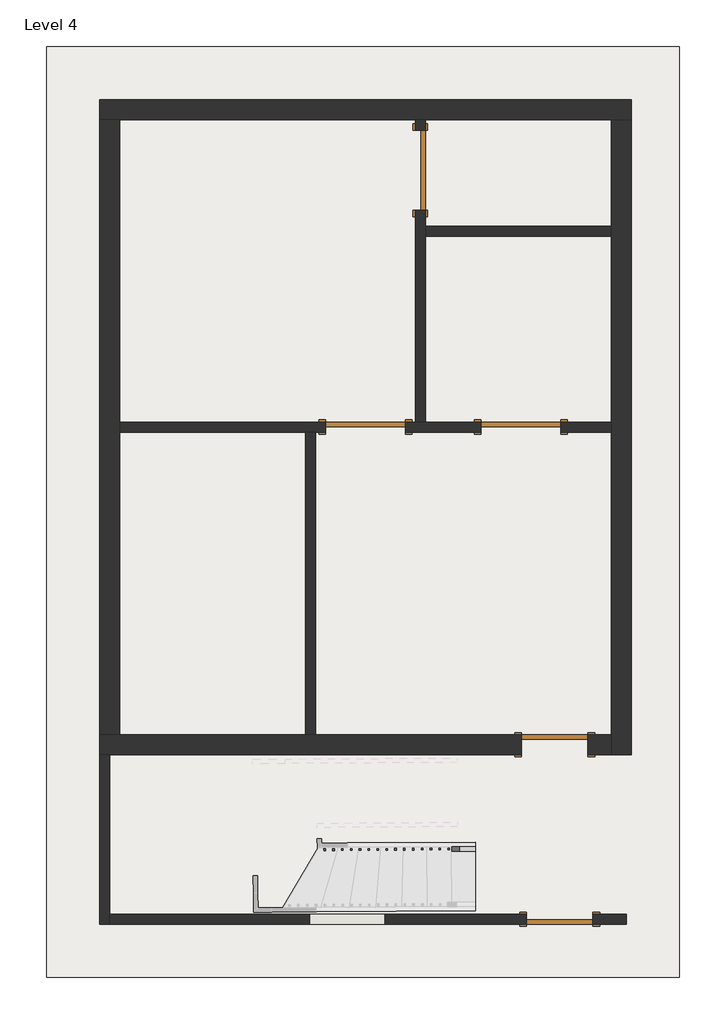
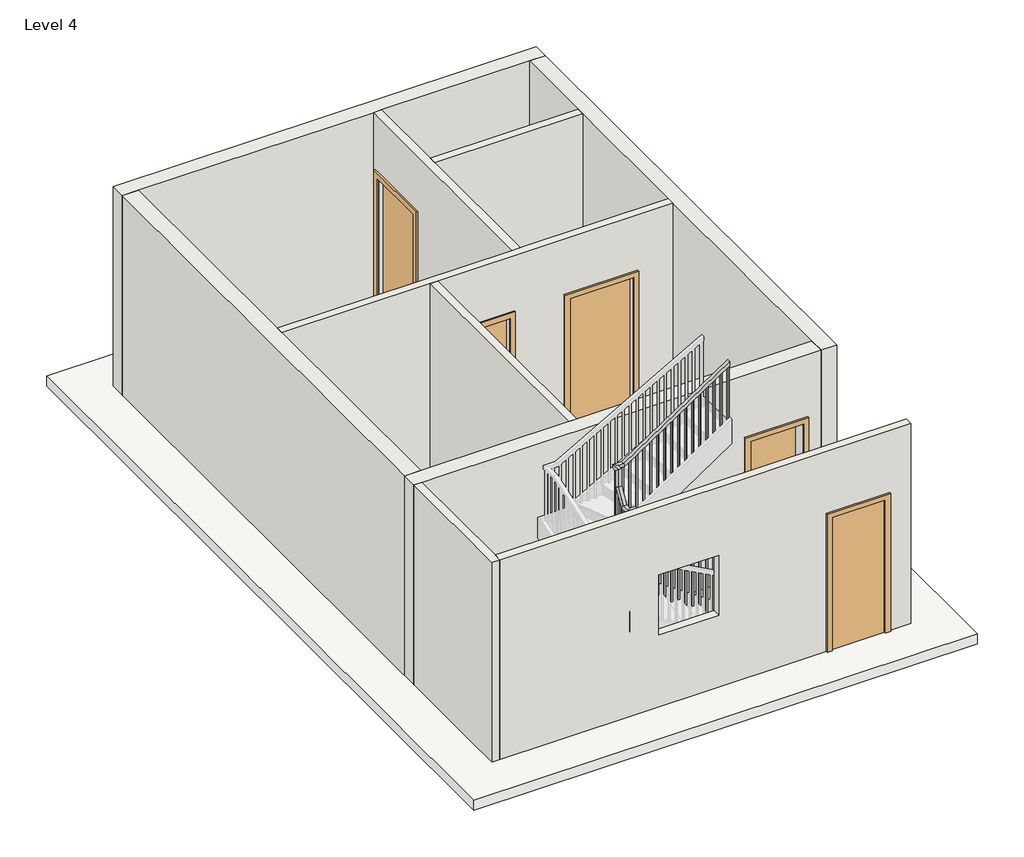
# One storey, part 1 of 2: 10 walls, 5 doors, 1 railing, 1 roof.
"""IFC4 building model written with IfcOpenShell, lengths in millimetres."""

from ifc_helpers import new_model, si_unit, frame, origin, place, context, project, spatial, polyline, outline, extrude, faceted_brep, transform, mapped, element, save
from components import door_a1484949, door_d8f5dbb5, door_e5f9f3c4, door_305aa2a5

model = new_model("IFC4")

# Units and contexts
model_context = context("Model", 3, world=origin())
ifc_project = project(units=[si_unit("LENGTHUNIT", "METRE", prefix="MILLI")], contexts=[model_context])

# Site, building, storey
site = spatial("IfcSite", under=ifc_project)
building = spatial("IfcBuilding", under=site)
storey = spatial("IfcBuildingStorey", under=building, Name="Level 4", Elevation=6400.8)

# Doors
placement = place(None, origin())
door_shape = door_a1484949(model_context)
element("IfcDoor", 1, ObjectType="Single-Flush : 30\" x 80\"", at=placement, inside=storey, context=model_context, shape_type="MappedRepresentation", body=[
    mapped(door_shape, transform((792.5410386, -2372.0109248, 6400.8), x_axis=(1.0, 0.0, 0.0), y_axis=(0.0, 1.0, 0.0), z_axis=(0.0, 0.0, 1.0))),
])
door_2_shape = door_d8f5dbb5(model_context)
element("IfcDoor", 2, ObjectType="Single-Flush : 30\" x 80\"", at=placement, inside=storey, context=model_context, shape_type="MappedRepresentation", body=[
    mapped(door_2_shape, transform((849.6910386, -4372.2609248, 6400.8), x_axis=(-1.0, 0.0, 0.0), y_axis=(0.0, -1.0, 0.0), z_axis=(0.0, 0.0, 1.0))),
])
door_3_shape = door_e5f9f3c4(model_context)
element("IfcDoor", 3, ObjectType="Single-Flush : 36\" x 84\"", at=placement, inside=storey, context=model_context, shape_type="MappedRepresentation", body=[
    mapped(door_3_shape, transform((-750.5089614, 4209.7640752, 6400.8), x_axis=(0.0, -1.0, 0.0), y_axis=(1.0, 0.0, 0.0), z_axis=(0.0, 0.0, 1.0))),
])
door_4_shape = door_305aa2a5(model_context)
element("IfcDoor", 4, ObjectType="Single-Flush : 36\" x 84\"", at=placement, inside=storey, context=model_context, shape_type="MappedRepresentation", body=[
    mapped(door_4_shape, transform((402.0160386, 1266.5390752, 6400.8), x_axis=(-1.0, 0.0, 0.0), y_axis=(0.0, -1.0, 0.0), z_axis=(0.0, 0.0, 1.0))),
])
element("IfcDoor", 5, ObjectType="Single-Flush : 36\" x 84\"", at=placement, inside=storey, context=model_context, shape_type="MappedRepresentation", body=[
    mapped(door_4_shape, transform((-1379.1589614, 1266.5390752, 6400.8), x_axis=(-1.0, 0.0, 0.0), y_axis=(0.0, -1.0, 0.0), z_axis=(0.0, 0.0, 1.0))),
])

# Railing
element("IfcRailing", 6, ObjectType="Handrail - Rectangular", at=placement, inside=storey, context=model_context, shape_type="SolidModel", body=[
    faceted_brep([(-120.3816305, -3590.4209536, 7484.5333333), (-120.3816305, -3590.4209536, 7423.3630107), (-120.6930289, -3539.621908, 7423.3630107), (-120.6930289, -3539.621908, 7484.5333333), (-1854.5612186, -3601.0514854, 8647.8182998), (-1905.3602642, -3601.3628839, 8620.7238978), (-1905.6716627, -3550.5638383, 8620.7238978), (-1854.8726171, -3550.2524399, 8647.8182998), (-1854.5612186, -3601.0514854, 8870.0829276), (-1905.3602642, -3601.3628839, 8819.2829276), (-1905.6716627, -3550.5638383, 8819.2829276), (-1854.8726171, -3550.2524399, 8870.0829276), (-1981.5588325, -3601.8299816, 8870.0829276), (-1981.5588325, -3601.8299816, 8819.2829276), (-1931.0711854, -3550.7195376, 8819.2829276), (-1931.0711854, -3550.7195376, 8870.0829276), (-1982.3373287, -3474.8323677, 8870.0829276), (-1982.5128182, -3446.2044317, 8819.2829276), (-1931.7137726, -3445.8930332, 8819.2829276), (-1931.5382832, -3474.5209692, 8870.0829276), (-1983.1158249, -3347.8347538, 9079.8434812), (-1983.4272234, -3297.0357082, 9065.6632575), (-1932.6281778, -3296.7243097, 9065.6632575), (-1932.3167793, -3347.5233553, 9079.8434812), (-1983.1158249, -3347.8347538, 9351.2951436), (-1983.4272234, -3297.0357082, 9300.4951436), (-1932.6281778, -3296.7243097, 9300.4951436), (-1932.3167793, -3347.5233553, 9351.2951436), (-1983.8943211, -3220.8371398, 9351.2951436), (-1983.8943211, -3220.8371398, 9300.4951436), (-1932.783877, -3271.3247869, 9300.4951436), (-1932.783877, -3271.3247869, 9351.2951436), (-1856.8967072, -3220.0586437, 9351.2951436), (-1841.6341703, -3219.9650842, 9300.4951436), (-1841.3227719, -3270.7641298, 9300.4951436), (-1856.5853087, -3270.8576892, 9351.2951436), (-324.9523945, -3210.6678153, 10363.2), (-324.6409961, -3261.4668609, 10363.2), (-324.6409961, -3261.4668609, 10302.3185401), (-324.9523945, -3210.6678153, 10302.3185401)], [[[0, 1, 2, 3]], [[1, 0, 4, 5]], [[2, 1, 5, 6]], [[3, 2, 6, 7]], [[0, 3, 7, 4]], [[5, 4, 8, 9]], [[6, 5, 9, 10]], [[7, 6, 10, 11]], [[4, 7, 11, 8]], [[9, 8, 12, 13]], [[10, 9, 13, 14]], [[11, 10, 14, 15]], [[8, 11, 15, 12]], [[13, 12, 16, 17]], [[14, 13, 17, 18]], [[15, 14, 18, 19]], [[12, 15, 19, 16]], [[17, 16, 20, 21]], [[18, 17, 21, 22]], [[19, 18, 22, 23]], [[16, 19, 23, 20]], [[21, 20, 24, 25]], [[22, 21, 25, 26]], [[23, 22, 26, 27]], [[20, 23, 27, 24]], [[25, 24, 28, 29]], [[26, 25, 29, 30]], [[27, 26, 30, 31]], [[24, 27, 31, 28]], [[29, 28, 32, 33]], [[30, 29, 33, 34]], [[31, 30, 34, 35]], [[28, 31, 35, 32]], [[36, 37, 38, 39]], [[33, 32, 36, 39]], [[34, 33, 39, 38]], [[35, 34, 38, 37]], [[32, 35, 37, 36]]]),
    extrude(outline(polyline([(222.3085098, -19.05), (234.8914903, 0.0), (1246.1854534, 0.0), (1246.1854534, -19.05), (222.3085098, -19.05)])), frame((-342.2360746, -3245.6994205, 10525.6521201), z_axis=(-0.00612989118043648, 0.9999812120405643, 0.0), x_axis=(0.0, 0.0, -1.0)), (0.0, 0.0, 1.0), 19.05),
    extrude(outline(polyline([(222.3085098, -19.0499999), (234.8914902, 0.0), (1179.0762243, 0.0), (1179.0762243, -19.0499999), (222.3085098, -19.0499999)])), frame((-443.8341657, -3246.3222175, 10458.542891), z_axis=(-0.00612989118043648, 0.9999812120405643, 0.0), x_axis=(0.0, 0.0, -1.0)), (0.0, 0.0, 1.0), 19.05),
    extrude(outline(polyline([(222.3085098, -19.05), (234.8914902, 0.0), (1111.9669952, 0.0), (1111.9669952, -19.05), (222.3085098, -19.05)])), frame((-545.4322569, -3246.9450144, 10391.4336619), z_axis=(-0.00612989118043648, 0.9999812120405643, 0.0), x_axis=(0.0, 0.0, -1.0)), (0.0, 0.0, 1.0), 19.05),
    extrude(outline(polyline([(222.3085098, -19.05), (234.8914902, 0.0), (1214.1910995, 0.0), (1214.1910995, -19.05), (222.3085098, -19.05)])), frame((-647.030348, -3247.5678114, 10324.3244328), z_axis=(-0.00612989118043648, 0.9999812120405643, 0.0), x_axis=(0.0, 0.0, -1.0)), (0.0, 0.0, 1.0), 19.05),
    extrude(outline(polyline([(222.3085098, -19.05), (234.8914902, 0.0), (1147.0818704, 0.0), (1147.0818704, -19.05), (222.3085098, -19.05)])), frame((-748.6284392, -3248.1906083, 10257.2152037), z_axis=(-0.00612989118043648, 0.9999812120405643, 0.0), x_axis=(0.0, 0.0, -1.0)), (0.0, 0.0, 1.0), 19.05),
    extrude(outline(polyline([(222.3085098, -19.05), (234.8914902, 0.0), (1079.9726413, 0.0), (1079.9726413, -19.05), (222.3085098, -19.05)])), frame((-850.2265303, -3248.8134053, 10190.1059746), z_axis=(-0.00612989118043648, 0.9999812120405643, 0.0), x_axis=(0.0, 0.0, -1.0)), (0.0, 0.0, 1.0), 19.05),
    extrude(outline(polyline([(222.3085098, -19.05), (234.8914902, 0.0), (1182.1967455, 0.0), (1182.1967455, -19.05), (222.3085098, -19.05)])), frame((-951.8246215, -3249.4362022, 10122.9967455), z_axis=(-0.00612989118043648, 0.9999812120405643, 0.0), x_axis=(0.0, 0.0, -1.0)), (0.0, 0.0, 1.0), 19.05),
    extrude(outline(polyline([(222.3085097, -19.05), (234.8914902, 0.0), (1115.0875164, 0.0), (1115.0875164, -19.05), (222.3085097, -19.05)])), frame((-1053.4227126, -3250.0589992, 10055.8875164), z_axis=(-0.00612989118043648, 0.9999812120405643, 0.0), x_axis=(0.0, 0.0, -1.0)), (0.0, 0.0, 1.0), 19.05),
    extrude(outline(polyline([(222.3085097, -19.0499999), (234.8914902, 0.0), (1047.9782873, 0.0), (1047.9782873, -19.0499999), (222.3085097, -19.0499999)])), frame((-1155.0208037, -3250.6817961, 9988.7782873), z_axis=(-0.00612989118043648, 0.9999812120405643, 0.0), x_axis=(0.0, 0.0, -1.0)), (0.0, 0.0, 1.0), 19.05),
    extrude(outline(polyline([(222.3085097, -19.05), (234.8914902, 0.0), (1150.2023915, 0.0), (1150.2023915, -19.05), (222.3085097, -19.05)])), frame((-1256.6188949, -3251.304593, 9921.6690582), z_axis=(-0.00612989118043648, 0.9999812120405643, 0.0), x_axis=(0.0, 0.0, -1.0)), (0.0, 0.0, 1.0), 19.05),
    extrude(outline(polyline([(222.3085098, -19.05), (234.8914903, 0.0), (1083.0931625, 0.0), (1083.0931625, -19.05), (222.3085098, -19.05)])), frame((-1358.216986, -3251.92739, 9854.5598292), z_axis=(-0.00612989118043648, 0.9999812120405643, 0.0), x_axis=(0.0, 0.0, -1.0)), (0.0, 0.0, 1.0), 19.05),
    extrude(outline(polyline([(222.3085098, -19.05), (234.8914903, 0.0), (1185.3172668, 0.0), (1185.3172668, -19.05), (222.3085098, -19.05)])), frame((-1459.8150772, -3252.5501869, 9787.4506001), z_axis=(-0.00612989118043648, 0.9999812120405643, 0.0), x_axis=(0.0, 0.0, -1.0)), (0.0, 0.0, 1.0), 19.05),
    extrude(outline(polyline([(222.3085098, -19.05), (234.8914903, 0.0), (1118.2080377, 0.0), (1118.2080377, -19.05), (222.3085098, -19.05)])), frame((-1561.4131683, -3253.1729839, 9720.341371), z_axis=(-0.00612989118043648, 0.9999812120405643, 0.0), x_axis=(0.0, 0.0, -1.0)), (0.0, 0.0, 1.0), 19.05),
    extrude(outline(polyline([(222.3085098, -19.05), (234.8914902, 0.0), (1051.0988086, 0.0), (1051.0988086, -19.05), (222.3085098, -19.05)])), frame((-1663.0112595, -3253.7957808, 9653.2321419), z_axis=(-0.00612989118043648, 0.9999812120405643, 0.0), x_axis=(0.0, 0.0, -1.0)), (0.0, 0.0, 1.0), 19.05),
    extrude(outline(polyline([(222.3085098, -19.05), (234.8914902, 0.0), (1153.3229128, 0.0), (1153.3229128, -19.05), (222.3085098, -19.05)])), frame((-1764.6093506, -3254.4185778, 9586.1229128), z_axis=(-0.00612989118043648, 0.9999812120405643, 0.0), x_axis=(0.0, 0.0, -1.0)), (0.0, 0.0, 1.0), 19.05),
    extrude(outline(polyline([(222.3085098, -19.05), (234.8914902, 0.0), (1086.2136837, 0.0), (1086.2136837, -19.05), (222.3085098, -19.05)])), frame((-1866.2074418, -3255.0413747, 9519.0136837), z_axis=(-0.00612989118043648, 0.9999812120405643, 0.0), x_axis=(0.0, 0.0, -1.0)), (0.0, 0.0, 1.0), 19.05),
    extrude(outline(polyline([(-1948.6001916, -3280.94692), (-1967.6498337, -3281.0636944), (-1967.7666081, -3262.0140523), (-1948.716966, -3261.8972779), (-1948.6001916, -3280.94692)])), frame((0.0, 0.0, 8263.4666667), z_axis=(0.0, 0.0, 1.0), x_axis=(1.0, 0.0, 0.0)), (0.0, 0.0, 1.0), 1037.0284769),
    extrude(outline(polyline([(244.3320415, -19.05), (212.8679585, 0.0), (1074.2735921, 0.0), (1074.2735921, -19.05), (244.3320415, -19.05)])), frame((-1967.1438111, -3363.6121435, 9168.4069254), z_axis=(0.9999812120405644, 0.006129891180436036, 0.0), x_axis=(0.0, 0.0, -1.0)), (0.0, 0.0, 1.0), 19.05),
    extrude(outline(polyline([(244.3320415, -19.05), (212.8679585, 0.0), (1075.7984825, 0.0), (1075.7984825, -19.05), (244.3320415, -19.05)])), frame((-1966.5210142, -3465.2102346, 9000.5984825), z_axis=(0.9999812120405644, 0.006129891180436036, 0.0), x_axis=(0.0, 0.0, -1.0)), (0.0, 0.0, 1.0), 19.05),
    extrude(outline(polyline([(-1939.8365364, -3566.6485675), (-1939.719762, -3585.6982096), (-1958.7694041, -3585.814984), (-1958.8861785, -3566.7653419), (-1939.8365364, -3566.6485675)])), frame((0.0, 0.0, 7755.4666667), z_axis=(0.0, 0.0, 1.0), x_axis=(1.0, 0.0, 0.0)), (0.0, 0.0, 1.0), 1063.816261),
    extrude(outline(polyline([(234.9892351, -19.05), (222.2107648, 0.0), (1224.4109792, 0.0), (1224.4109792, -19.05), (234.9892351, -19.05)])), frame((-1857.171313, -3585.1921871, 8810.5443125), z_axis=(-0.006129891180436334, 0.9999812120405643, 0.0), x_axis=(0.0, 0.0, -1.0)), (0.0, 0.0, 1.0), 19.05),
    extrude(outline(polyline([(234.9892352, -19.05), (222.2107649, 0.0), (1156.259138, 0.0), (1156.259138, -19.05), (234.9892352, -19.05)])), frame((-1755.5732218, -3584.5693901, 8742.3924713), z_axis=(-0.006129891180436334, 0.9999812120405643, 0.0), x_axis=(0.0, 0.0, -1.0)), (0.0, 0.0, 1.0), 19.05),
    extrude(outline(polyline([(234.9892351, -19.05), (222.2107649, 0.0), (1257.44063, 0.0), (1257.44063, -19.05), (234.9892351, -19.05)])), frame((-1653.9751307, -3583.9465932, 8674.24063), z_axis=(-0.006129891180436334, 0.9999812120405643, 0.0), x_axis=(0.0, 0.0, -1.0)), (0.0, 0.0, 1.0), 19.05),
    extrude(outline(polyline([(234.9892351, -19.05), (222.2107649, 0.0), (1189.2887887, 0.0), (1189.2887887, -19.05), (234.9892351, -19.05)])), frame((-1552.3770395, -3583.3237962, 8606.0887887), z_axis=(-0.006129891180436334, 0.9999812120405643, 0.0), x_axis=(0.0, 0.0, -1.0)), (0.0, 0.0, 1.0), 19.05),
    extrude(outline(polyline([(234.9892351, -19.05), (222.2107649, 0.0), (1290.4702807, 0.0), (1290.4702807, -19.05), (234.9892351, -19.05)])), frame((-1450.7789484, -3582.7009993, 8537.9369474), z_axis=(-0.006129891180436334, 0.9999812120405643, 0.0), x_axis=(0.0, 0.0, -1.0)), (0.0, 0.0, 1.0), 19.05),
    extrude(outline(polyline([(234.9892351, -19.0499999), (222.2107649, 0.0), (1222.3184394, 0.0), (1222.3184394, -19.0499999), (234.9892351, -19.0499999)])), frame((-1349.1808572, -3582.0782024, 8469.7851061), z_axis=(-0.006129891180436334, 0.9999812120405643, 0.0), x_axis=(0.0, 0.0, -1.0)), (0.0, 0.0, 1.0), 19.05),
    extrude(outline(polyline([(234.9892351, -19.05), (222.2107648, 0.0), (1154.1665981, 0.0), (1154.1665981, -19.05), (234.9892351, -19.05)])), frame((-1247.5827661, -3581.4554054, 8401.6332648), z_axis=(-0.006129891180436334, 0.9999812120405643, 0.0), x_axis=(0.0, 0.0, -1.0)), (0.0, 0.0, 1.0), 19.05),
    extrude(outline(polyline([(234.9892352, -19.05), (222.2107649, 0.0), (1255.3480903, 0.0), (1255.3480903, -19.05), (234.9892352, -19.05)])), frame((-1145.984675, -3580.8326085, 8333.4814236), z_axis=(-0.006129891180436334, 0.9999812120405643, 0.0), x_axis=(0.0, 0.0, -1.0)), (0.0, 0.0, 1.0), 19.05),
    extrude(outline(polyline([(234.9892351, -19.05), (222.2107649, 0.0), (1187.196249, 0.0), (1187.196249, -19.05), (234.9892351, -19.05)])), frame((-1044.3865838, -3580.2098115, 8265.3295823), z_axis=(-0.006129891180436334, 0.9999812120405643, 0.0), x_axis=(0.0, 0.0, -1.0)), (0.0, 0.0, 1.0), 19.05),
    extrude(outline(polyline([(234.9892351, -19.05), (222.2107649, 0.0), (1288.377741, 0.0), (1288.377741, -19.05), (234.9892351, -19.05)])), frame((-942.7884927, -3579.5870146, 8197.177741), z_axis=(-0.006129891180436334, 0.9999812120405643, 0.0), x_axis=(0.0, 0.0, -1.0)), (0.0, 0.0, 1.0), 19.05),
    extrude(outline(polyline([(234.9892351, -19.05), (222.2107649, 0.0), (1220.2258997, 0.0), (1220.2258997, -19.05), (234.9892351, -19.05)])), frame((-841.1904015, -3578.9642176, 8129.0258997), z_axis=(-0.006129891180436334, 0.9999812120405643, 0.0), x_axis=(0.0, 0.0, -1.0)), (0.0, 0.0, 1.0), 19.05),
    extrude(outline(polyline([(234.9892351, -19.05), (222.2107649, 0.0), (1152.0740584, 0.0), (1152.0740584, -19.05), (234.9892351, -19.05)])), frame((-739.5923104, -3578.3414207, 8060.8740584), z_axis=(-0.006129891180436334, 0.9999812120405643, 0.0), x_axis=(0.0, 0.0, -1.0)), (0.0, 0.0, 1.0), 19.05),
    extrude(outline(polyline([(234.9892351, -19.0499999), (222.2107648, 0.0), (1253.2555504, 0.0), (1253.2555504, -19.0499999), (234.9892351, -19.0499999)])), frame((-637.9942192, -3577.7186237, 7992.7222171), z_axis=(-0.006129891180436334, 0.9999812120405643, 0.0), x_axis=(0.0, 0.0, -1.0)), (0.0, 0.0, 1.0), 19.05),
    extrude(outline(polyline([(234.9892352, -19.05), (222.2107649, 0.0), (1185.1037092, 0.0), (1185.1037092, -19.05), (234.9892352, -19.05)])), frame((-536.3961281, -3577.0958268, 7924.5703759), z_axis=(-0.006129891180436334, 0.9999812120405643, 0.0), x_axis=(0.0, 0.0, -1.0)), (0.0, 0.0, 1.0), 19.05),
    extrude(outline(polyline([(234.9892351, -19.05), (222.2107649, 0.0), (1116.9518679, 0.0), (1116.9518679, -19.05), (234.9892351, -19.05)])), frame((-434.798037, -3576.4730299, 7856.4185346), z_axis=(-0.006129891180436334, 0.9999812120405643, 0.0), x_axis=(0.0, 0.0, -1.0)), (0.0, 0.0, 1.0), 19.05),
    extrude(outline(polyline([(234.9892351, -19.05), (222.2107649, 0.0), (1218.13336, 0.0), (1218.13336, -19.05), (234.9892351, -19.05)])), frame((-333.1999458, -3575.8502329, 7788.2666933), z_axis=(-0.006129891180436334, 0.9999812120405643, 0.0), x_axis=(0.0, 0.0, -1.0)), (0.0, 0.0, 1.0), 19.05),
    extrude(outline(polyline([(234.9892351, -19.05), (222.2107649, 0.0), (1149.9815187, 0.0), (1149.9815187, -19.05), (234.9892351, -19.05)])), frame((-231.6018547, -3575.227436, 7720.114852), z_axis=(-0.006129891180436334, 0.9999812120405643, 0.0), x_axis=(0.0, 0.0, -1.0)), (0.0, 0.0, 1.0), 19.05),
    extrude(outline(polyline([(-1948.7558908, -3255.5473972), (-1967.8055329, -3255.6641716), (-1967.9223073, -3236.6145296), (-1948.8726652, -3236.4977551), (-1948.7558908, -3255.5473972)])), frame((0.0, 0.0, 8263.4666667), z_axis=(0.0, 0.0, 1.0), x_axis=(1.0, 0.0, 0.0)), (0.0, 0.0, 1.0), 1037.0284769),
    extrude(outline(polyline([(-1946.8485752, -3566.6915513), (-1946.7318007, -3585.7411934), (-1965.7814428, -3585.8579679), (-1965.8982173, -3566.8083258), (-1946.8485752, -3566.6915513)])), frame((0.0, 0.0, 7755.4666667), z_axis=(0.0, 0.0, 1.0), x_axis=(1.0, 0.0, 0.0)), (0.0, 0.0, 1.0), 1063.816261),
    extrude(outline(polyline([(222.3085098, -19.05), (234.8914902, 0.0), (1245.1603832, 0.0), (1245.1603832, -19.05), (222.3085098, -19.05)])), frame((-343.7879502, -3245.7089335, 10524.6270499), z_axis=(-0.00612989118043648, 0.9999812120405643, 0.0), x_axis=(0.0, 0.0, -1.0)), (0.0, 0.0, 1.0), 19.05),
    extrude(outline(polyline([(234.9892351, -19.05), (222.2107648, 0.0), (1088.2189125, 0.0), (1088.2189125, -19.05), (234.9892351, -19.05)])), frame((-139.5285846, -3574.6630262, 7658.3522458), z_axis=(-0.006129891180436334, 0.9999812120405643, 0.0), x_axis=(0.0, 0.0, -1.0)), (0.0, 0.0, 1.0), 19.05),
])

# Roof
element("IfcRoof", 7, ObjectType="Generic - 12\"", at=placement, inside=storey, context=model_context, shape_type="SweptSolid", body=[
    extrude(outline(polyline([(-5036.7589614, 5628.9890752), (2221.2910386, 5628.9890752), (2221.2910386, -5039.0109248), (-5036.7589614, -5039.0109248), (-5036.7589614, 5628.9890752)])), frame((0.0, 0.0, 6248.4), z_axis=(0.0, 0.0, 1.0), x_axis=(1.0, 0.0, 0.0)), (0.0, 0.0, 1.0), 152.4),
])

# Walls
element("IfcWall", 8, ObjectType="4.5\"", at=placement, inside=storey, context=model_context, shape_type="Brep", body=[
    faceted_brep([(-807.6589614, 3752.5640752, 8534.4), (-807.6589614, 3752.5640752, 6400.8), (-807.6589614, 1323.6890752, 6400.8), (-807.6589614, 1323.6890752, 9448.8), (-807.6589614, 4790.7890752, 9448.8), (-807.6589614, 4790.7890752, 6400.8), (-807.6589614, 4666.9640752, 6400.8), (-807.6589614, 4666.9640752, 8534.4), (-693.3589614, 1323.6890752, 6400.8), (-693.3589614, 3457.2890752, 6400.8), (-693.3589614, 3571.5890752, 6400.8), (-693.3589614, 3752.5640752, 6400.8), (-693.3589614, 3752.5640752, 8534.4), (-693.3589614, 4666.9640752, 8534.4), (-693.3589614, 4666.9640752, 6400.8), (-693.3589614, 4790.7890752, 6400.8), (-693.3589614, 4790.7890752, 9448.8), (-693.3589614, 3571.5890752, 9448.8), (-693.3589614, 3457.2890752, 9448.8), (-693.3589614, 1323.6890752, 9448.8)], [[[0, 1, 2, 3, 4, 5, 6, 7]], [[8, 9, 10, 11, 12, 13, 14, 15, 16, 17, 18, 19]], [[6, 5, 15, 14]], [[2, 1, 11, 10, 9, 8]], [[5, 4, 16, 15]], [[3, 2, 8, 19]], [[12, 11, 1, 0]], [[13, 12, 0, 7]], [[14, 13, 7, 6]], [[4, 3, 19, 18, 17, 16]]]),
])
element("IfcWall", 9, ObjectType="4.5\"", at=placement, inside=storey, context=model_context, shape_type="SweptSolid", body=[
    extrude(outline(polyline([(-693.3589614, 3571.5890752), (1440.2410386, 3571.5890752), (1440.2410386, 3457.2890752), (-693.3589614, 3457.2890752), (-693.3589614, 3571.5890752)])), frame((0.0, 0.0, 6400.8), z_axis=(0.0, 0.0, 1.0), x_axis=(1.0, 0.0, 0.0)), (0.0, 0.0, 1.0), 3048.0),
])
element("IfcWall", 10, ObjectType="4.5\"", at=placement, inside=storey, context=model_context, shape_type="Brep", body=[
    faceted_brep([(-4198.5589614, 1209.3890752, 6400.8), (-2064.9589614, 1209.3890752, 6400.8), (-1950.6589614, 1209.3890752, 6400.8), (-1836.3589614, 1209.3890752, 6400.8), (-1836.3589614, 1209.3890752, 8534.4), (-921.9589614, 1209.3890752, 8534.4), (-921.9589614, 1209.3890752, 6400.8), (-55.1839614, 1209.3890752, 6400.8), (-55.1839614, 1209.3890752, 8534.4), (859.2160386, 1209.3890752, 8534.4), (859.2160386, 1209.3890752, 6400.8), (1440.2410386, 1209.3890752, 6400.8), (1440.2410386, 1209.3890752, 9448.8), (-1950.6589614, 1209.3890752, 9448.8), (-2064.9589614, 1209.3890752, 9448.8), (-4198.5589614, 1209.3890752, 9448.8), (-1836.3589614, 1323.6890752, 8534.4), (-1836.3589614, 1323.6890752, 6400.8), (-4198.5589614, 1323.6890752, 6400.8), (-4198.5589614, 1323.6890752, 9448.8), (-807.6589614, 1323.6890752, 9448.8), (-693.3589614, 1323.6890752, 9448.8), (1440.2410386, 1323.6890752, 9448.8), (1440.2410386, 1323.6890752, 6400.8), (859.2160386, 1323.6890752, 6400.8), (859.2160386, 1323.6890752, 8534.4), (-55.1839614, 1323.6890752, 8534.4), (-55.1839614, 1323.6890752, 6400.8), (-693.3589614, 1323.6890752, 6400.8), (-807.6589614, 1323.6890752, 6400.8), (-921.9589614, 1323.6890752, 6400.8), (-921.9589614, 1323.6890752, 8534.4)], [[[0, 1, 2, 3, 4, 5, 6, 7, 8, 9, 10, 11, 12, 13, 14, 15]], [[16, 17, 18, 19, 20, 21, 22, 23, 24, 25, 26, 27, 28, 29, 30, 31]], [[24, 23, 11, 10]], [[18, 17, 3, 2, 1, 0]], [[30, 29, 28, 27, 7, 6]], [[12, 11, 23, 22]], [[0, 15, 19, 18]], [[8, 7, 27, 26]], [[9, 8, 26, 25]], [[10, 9, 25, 24]], [[4, 3, 17, 16]], [[5, 4, 16, 31]], [[6, 5, 31, 30]], [[15, 14, 13, 12, 22, 21, 20, 19]]]),
])
element("IfcWall", 11, ObjectType="4.5\"", at=placement, inside=storey, context=model_context, shape_type="SweptSolid", body=[
    extrude(outline(polyline([(-2064.9589614, -2257.7109248), (-2064.9589614, 1209.3890752), (-1950.6589614, 1209.3890752), (-1950.6589614, -2257.7109248), (-2064.9589614, -2257.7109248)])), frame((0.0, 0.0, 6400.8), z_axis=(0.0, 0.0, 1.0), x_axis=(1.0, 0.0, 0.0)), (0.0, 0.0, 1.0), 3048.0),
])
element("IfcWall", 12, ObjectType="4.5\"", at=placement, inside=storey, context=model_context, shape_type="Brep", body=[
    faceted_brep([(-4427.1589614, -2486.3109248, 6400.8), (-4427.1589614, -4429.4109248, 6400.8), (-4427.1589614, -4429.4109248, 9448.8), (-4427.1589614, -2486.3109248, 9448.8), (-4312.8589614, -2486.3109248, 6400.8), (-4312.8589614, -2486.3109248, 9448.8), (-4312.8589614, -4315.1109248, 9448.8), (-4312.8589614, -4429.4109248, 9448.8), (-4312.8589614, -4429.4109248, 6400.8), (-4312.8589614, -4315.1109248, 6400.8)], [[[0, 1, 2, 3]], [[4, 5, 6, 7, 8, 9]], [[1, 0, 4, 9, 8]], [[3, 2, 7, 6, 5]], [[0, 3, 5, 4]], [[2, 1, 8, 7]]]),
])
element("IfcWall", 13, ObjectType="4.5\"", at=placement, inside=storey, context=model_context, shape_type="SweptSolid", body=[
    extrude(outline(polyline([(6400.8, -4312.8589614), (6400.8, 468.6910386), (8432.8, 468.6910386), (8432.8, 1230.6910386), (6400.8, 1230.6910386), (6400.8, 1611.6910386), (9448.8, 1611.6910386), (9448.8, -4312.8589614), (6400.8, -4312.8589614)]), holes=[polyline([(8412.3697748, -2020.5089614), (8412.3697748, -1156.9089614), (7497.9697748, -1156.9089614), (7497.9697748, -2020.5089614), (8412.3697748, -2020.5089614)])]), frame((0.0, -4429.4109248, 0.0), z_axis=(0.0, 1.0, 0.0), x_axis=(0.0, 0.0, 1.0)), (0.0, 0.0, 1.0), 114.3),
])
element("IfcWall", 14, ObjectType="9\"", at=placement, inside=storey, context=model_context, shape_type="Brep", body=[
    faceted_brep([(-4427.1589614, 4790.7890752, 6400.8), (-4198.5589614, 4790.7890752, 6400.8), (-807.6589614, 4790.7890752, 6400.8), (-693.3589614, 4790.7890752, 6400.8), (1440.2410386, 4790.7890752, 6400.8), (1668.8410386, 4790.7890752, 6400.8), (1668.8410386, 4790.7890752, 9448.8), (1440.2410386, 4790.7890752, 9448.8), (-693.3589614, 4790.7890752, 9448.8), (-807.6589614, 4790.7890752, 9448.8), (-4198.5589614, 4790.7890752, 9448.8), (-4427.1589614, 4790.7890752, 9448.8), (-4427.1589614, 5019.3890752, 6400.8), (-4427.1589614, 5019.3890752, 9448.8), (1668.8410386, 5019.3890752, 9448.8), (1668.8410386, 5019.3890752, 6400.8)], [[[0, 1, 2, 3, 4, 5, 6, 7, 8, 9, 10, 11]], [[12, 13, 14, 15]], [[5, 4, 3, 2, 1, 0, 12, 15]], [[6, 5, 15, 14]], [[0, 11, 13, 12]], [[11, 10, 9, 8, 7, 6, 14, 13]]]),
])
element("IfcWall", 15, ObjectType="9\"", at=placement, inside=storey, context=model_context, shape_type="Brep", body=[
    faceted_brep([(1440.2410386, 4790.7890752, 6400.8), (1440.2410386, 3571.5890752, 6400.8), (1440.2410386, 3457.2890752, 6400.8), (1440.2410386, 1323.6890752, 6400.8), (1440.2410386, 1209.3890752, 6400.8), (1440.2410386, -2257.7109248, 6400.8), (1440.2410386, -2486.3109248, 6400.8), (1440.2410386, -2486.3109248, 9448.8), (1440.2410386, -2257.7109248, 9448.8), (1440.2410386, 1209.3890752, 9448.8), (1440.2410386, 1323.6890752, 9448.8), (1440.2410386, 3457.2890752, 9448.8), (1440.2410386, 3571.5890752, 9448.8), (1440.2410386, 4790.7890752, 9448.8), (1668.8410386, 4790.7890752, 6400.8), (1668.8410386, 4790.7890752, 9448.8), (1668.8410386, -2486.3109248, 9448.8), (1668.8410386, -2486.3109248, 6400.8)], [[[0, 1, 2, 3, 4, 5, 6, 7, 8, 9, 10, 11, 12, 13]], [[14, 15, 16, 17]], [[6, 5, 4, 3, 2, 1, 0, 14, 17]], [[0, 13, 15, 14]], [[7, 6, 17, 16]], [[13, 12, 11, 10, 9, 8, 7, 16, 15]]]),
])
element("IfcWall", 16, ObjectType="9\"", at=placement, inside=storey, context=model_context, shape_type="Brep", body=[
    faceted_brep([(1440.2410386, -2257.7109248, 6400.8), (1173.5410386, -2257.7109248, 6400.8), (1173.5410386, -2257.7109248, 8432.8), (411.5410386, -2257.7109248, 8432.8), (411.5410386, -2257.7109248, 6400.8), (-1950.6589614, -2257.7109248, 6400.8), (-2064.9589614, -2257.7109248, 6400.8), (-4198.5589614, -2257.7109248, 6400.8), (-4427.1589614, -2257.7109248, 6400.8), (-4427.1589614, -2257.7109248, 9448.8), (-4198.5589614, -2257.7109248, 9448.8), (-2064.9589614, -2257.7109248, 9448.8), (-1950.6589614, -2257.7109248, 9448.8), (1440.2410386, -2257.7109248, 9448.8), (1173.5410386, -2486.3109248, 8432.8), (1173.5410386, -2486.3109248, 6400.8), (1440.2410386, -2486.3109248, 6400.8), (1440.2410386, -2486.3109248, 9448.8), (-4312.8589614, -2486.3109248, 9448.8), (-4427.1589614, -2486.3109248, 9448.8), (-4427.1589614, -2486.3109248, 6400.8), (-4312.8589614, -2486.3109248, 6400.8), (411.5410386, -2486.3109248, 6400.8), (411.5410386, -2486.3109248, 8432.8)], [[[0, 1, 2, 3, 4, 5, 6, 7, 8, 9, 10, 11, 12, 13]], [[14, 15, 16, 17, 18, 19, 20, 21, 22, 23]], [[16, 15, 1, 0]], [[22, 21, 20, 8, 7, 6, 5, 4]], [[0, 13, 17, 16]], [[9, 8, 20, 19]], [[2, 1, 15, 14]], [[3, 2, 14, 23]], [[4, 3, 23, 22]], [[13, 12, 11, 10, 9, 19, 18, 17]]]),
])
element("IfcWall", 17, ObjectType="9\"", at=placement, inside=storey, context=model_context, shape_type="Brep", body=[
    faceted_brep([(-4198.5589614, -2257.7109248, 6400.8), (-4198.5589614, 1209.3890752, 6400.8), (-4198.5589614, 1323.6890752, 6400.8), (-4198.5589614, 4790.7890752, 6400.8), (-4198.5589614, 4790.7890752, 9448.8), (-4198.5589614, 1323.6890752, 9448.8), (-4198.5589614, 1209.3890752, 9448.8), (-4198.5589614, -2257.7109248, 9448.8), (-4427.1589614, -2257.7109248, 6400.8), (-4427.1589614, -2257.7109248, 9448.8), (-4427.1589614, 4790.7890752, 9448.8), (-4427.1589614, 4790.7890752, 6400.8)], [[[0, 1, 2, 3, 4, 5, 6, 7]], [[8, 9, 10, 11]], [[3, 2, 1, 0, 8, 11]], [[0, 7, 9, 8]], [[4, 3, 11, 10]], [[7, 6, 5, 4, 10, 9]]]),
])

save(model, "model.ifc")

# Revit data of these elements
# Type "Single-Flush : 30\" x 80\""
#   Type Mark = "5"
#   Construction Type Id = "MDOOR"
#   Assembly Code = "C1020"
#   Analytic Construction = "Metal"
#   Thickness = 0' - 2"
#   Heat Transfer Coefficient (U) = 0.651978 BTU/(h·ft²·°F)
#   Height = 6' - 8"
#   Trim Projection Ext = 0' - 1"
#   Trim Projection Int = 0' - 1"
#   Trim Width = 0' - 3"
#   Width = 2' - 6"
#   Define Thermal Properties by = 1
#   Define Thermal Properties by = 1
#   Door Material = Door - Panel
#   Frame Material = Door - Frame
#   Visual Light Transmittance = 0
#   Solar Heat Gain Coefficient = 0
#   Function = (empty or 0)
#   Wall Closure = (empty or 0)
# Type "Single-Flush : 36\" x 84\""
#   Type Mark = "1"
#   Construction Type Id = "MDOOR"
#   Assembly Code = "C1020"
#   Analytic Construction = "Metal"
#   Thickness = 0' - 2"
#   Heat Transfer Coefficient (U) = 0.651978 BTU/(h·ft²·°F)
#   Height = 7' - 0"
#   Trim Projection Ext = 0' - 1"
#   Trim Projection Int = 0' - 1"
#   Trim Width = 0' - 3"
#   Width = 3' - 0"
#   Define Thermal Properties by = 1
#   Define Thermal Properties by = 1
#   Door Material = Door - Panel
#   Frame Material = Door - Frame
#   Visual Light Transmittance = 0
#   Solar Heat Gain Coefficient = 0
#   Function = (empty or 0)
#   Wall Closure = (empty or 0)
# Type "Handrail - Rectangular"
#   Assembly Code = "C2010400"
#   built-in parameter 1008612 = 0.0416667 (stored number, unit not read)
#   built-in parameter 1008611 = 0.0416667 (stored number, unit not read)
#   built-in parameter 1008609 = 0.333333 (stored number, unit not read)
#   built-in parameter 1008604 = 0.166667 (stored number, unit not read)
#   built-in parameter 1008603 = 0.166667 (stored number, unit not read)
#   Railing Height = 3' - 0"
#   built-in parameter 1008630 = 2
#   built-in parameter 1008610 = 2
#   built-in parameter 1008618 = Baluster - Square : 3/4"
# Type "Generic - 12\""
#   Assembly Code = "B1020"
#   Layers, outside or top first: 0' - 6" no material (function 1)
# Type "4.5\""
#   Assembly Code = "B2010"
#   Layers, outside or top first: 0' - 4 1/2" no material (function 1)
# Type "9\""
#   Assembly Code = "B2010"
#   Layers, outside or top first: 0' - 9" no material (function 1)
# Elements 1, 2 (IfcDoor, "Single-Flush : 30\" x 80\"")
#   Phase Created = New Construction
#   Materials on its faces: "Door - Frame", "Door - Panel"
# Elements 3, 4, 5 (IfcDoor, "Single-Flush : 36\" x 84\"")
#   Phase Created = New Construction
#   Materials on its faces: "Door - Frame", "Door - Panel"
# Element 6 (IfcRailing, "Handrail - Rectangular")
#   Phase Created = New Construction
# Element 7 (IfcRoof, "Generic - 12\"")
#   built-in parameter 1001705 = 21 (stored number, unit not read)
#   built-in parameter 1001701 = -0.5 (stored number, unit not read)
#   built-in parameter 1001710 = 33615
#   Phase Created = New Construction
#   Materials on its faces: "Default Roof"
# Elements 8, 9, 10, 11 (IfcWall, "4.5\"")
#   Top Offset = 0' - 0"
#   Base Offset = 0' - 0"
#   Unconnected Height = 10' - 0"
#   wall height = 10' - 0"
#   Phase Created = New Construction
#   Base Constraint = Level 4
#   Materials on its faces: "Default Wall"
# Elements 12, 13 (IfcWall, "4.5\"")
#   Top Offset = 0' - 0"
#   Base Offset = 0' - 0"
#   Unconnected Height = 10' - 0"
#   wall height = 10' - 0"
#   Phase Created = New Construction
#   Base Constraint = Level 4
#   Materials on its faces: "Default Wall", "Door - Frame"
# Elements 14, 15, 16, 17 (IfcWall, "9\"")
#   Top Offset = 0' - 0"
#   Base Offset = 0' - 0"
#   Unconnected Height = 10' - 0"
#   wall height = 10' - 0"
#   Phase Created = New Construction
#   Base Constraint = Level 4
#   Materials on its faces: "Default Wall", "Door - Frame"
# Materials
#   "Door - Panel": class "Wood", colour RGB 210 159 95, transparency 0, Cost = 0
#   "Door - Frame": colour RGB 118 70 51, transparency 0, Cost = 0
#   "Default Roof": colour RGB 88 101 114, transparency 0, Cost = 0
#   "Default Wall": colour RGB 128 128 128, transparency 0, Cost = 0
